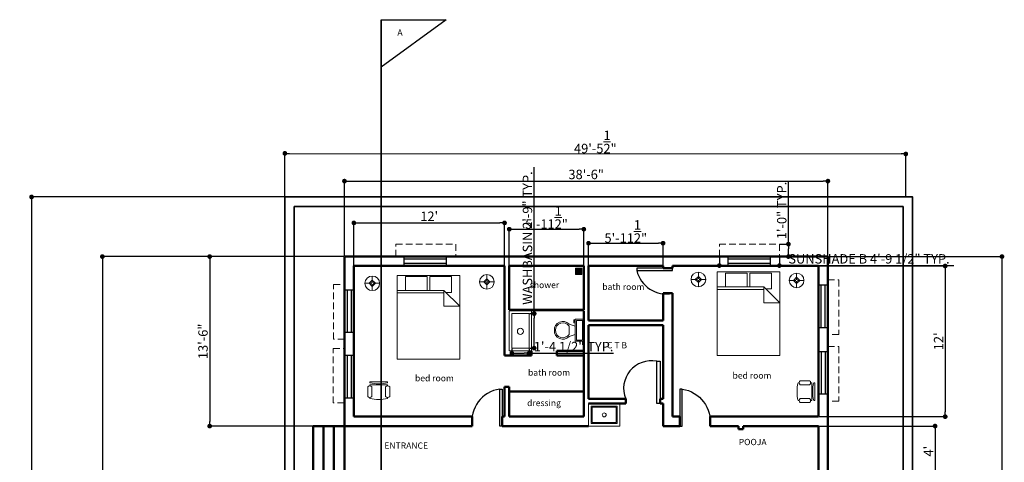
# Model space of a CAD drawing. Units: inches. Extents: x 2050 to 6806, y 2092 to 5743.
# Tile 3 of 8: x 2050 to 2991, y 2706 to 3129. Entities that reach past the tile are written whole.
import ezdxf

# ---------------------------------------------------------------- set-up
doc = ezdxf.new("R2010")
doc.units = ezdxf.units.IN
doc.linetypes.add('HIDDEN', pattern=[9.525, 6.35, -3.175])
for name, color, linetype, lineweight in [('A-ANNO-DIMS', 2, 'Continuous', 18), ('A-ANNO-SYMB', 1, 'Continuous', 25), ('A-AREA-IDEN', 7, 'Continuous', 18), ('A-DOOR', 2, 'Continuous', 25), ('A-FLOR-FIXT', 4, 'Continuous', 18), ('A-FLOR-OVHD', 30, 'HIDDEN', 18), ('A-FURN', 5, 'Continuous', 18), ('A-GLAZ', 6, 'Continuous', 25), ('A-WALL', 7, 'Continuous', 50), ('C-PROP', 90, 'Continuous', 35)]:
    doc.layers.add(name, color=color, linetype=linetype, lineweight=lineweight)
doc.styles.get("Standard").update_dxf_attribs({"font": 'arial.ttf'})
doc.dimstyles.new('ISO-25', dxfattribs={"dimtxt": 9, "dimasz": 4.5, "dimexe": 1.25, "dimexo": 0.625, "dimtad": 1, "dimdec": 1, "dimlunit": 4, "dimtxsty": 'Standard', "dimblk": 'DOT', "dimcen": 2.5, "dimadec": 0, "dimazin": 0, "dimtfac": 1, "dimtdec": 1, "dimtmove": 0, "dimatfit": 3, "dimldrblk": 'ARCHTICK', "dimfxl": 1, "dimarcsym": 0})

# ---------------------------------------------------------------- blocks, each defined once
blk = doc.blocks.new('*U4')
for p, q in [((-10, -8.5), (-8, -8.5)), ((-10, -9.5), (-10, -8.5)), ((-8, -8.5), (-8, -8)), ((-7, -8), (-7, -9.5)), ((-4, -8), (-6, -14)), ((4, -8), (6, -14)), ((9.5, -6), (9.5, -2)), ((-7, -9.5), (-10, -9.5)), ((4, -14), (-4, -14))]:
    blk.add_line(p, q)
blk.add_lwpolyline([(10.5, -8), (10.5, 0), (-10.5, 0), (-10.5, -8)], close=True)
for points in [[(-9.5, -2), (-9.5, -6)], [(8.5, -1), (-8.5, -1)], [(-8.5, -7), (8.5, -7)]]:
    blk.add_lwpolyline(points)
for centre, radius, start, end in [((-8.625, -1.875), 0.8839, 81.8699, 188.1301), ((-8.625, -6.125), 0.8839, 171.869898, 278.1301), ((8.625, -1.875), 0.8839, 351.8699, 98.1301), ((8.625, -6.125), 0.8839, 261.8699, 8.1301), ((-0.4772, -19.9188), 8.0953, 133.01722, 273.38), ((0.0374, -19.8731), 7.127, 124.50543, 269.7), ((-0.0373, -19.8731), 7.127, 270.3, 55.4946), ((0.4773, -19.9188), 8.0953, 266.62, 46.9828)]:
    blk.add_arc(centre, radius, start, end)
blk = doc.blocks.new('Bed - Queen')
for p, q in [((0, -80.00003), (0, 0)), ((0, 0), (59.99999, 0)), ((59.99999, 0), (59.99999, -80.00003)), ((7.99999, -1.2), (28.79998, -1.2)), ((7.99999, -14.4), (7.99999, -1.2)), ((28.79998, -1.2), (28.79998, -14.4)), ((31.19999, -1.2), (51.99999, -1.2)), ((31.19999, -14.4), (31.19999, -1.2)), ((51.99999, -1.2), (51.99999, -16.4)), ((0, -14.4), (44.8, -14.4)), ((44.8, -16.8), (0, -16.8)), ((59.99999, -29.6), (44.8, -14.4)), ((44.8, -14.4), (44.8, -29.6)), ((51.99999, -16.4), (46.79936, -16.4)), ((44.8, -29.6), (59.99999, -29.6)), ((59.99999, -80.00003), (0, -80.00003))]:
    blk.add_line(p, q)
blk = doc.blocks.new('Lamp - Table')
for p, q in [((-1, 0), (-7, 0)), ((0, 3), (-3, 0)), ((-3, 0), (0, -3)), ((0, 7), (0, 1)), ((3, 0), (0, 3)), ((0, -3), (3, 0)), ((1, 0), (7, 0)), ((0, -1), (0, -7))]:
    blk.add_line(p, q)
for radius in [7, 1]:
    blk.add_circle((0, 0), radius)
blk = doc.blocks.new('Chair - Desk')
for p, q in [((-8.5, 0), (-8.5, -1)), ((-8.5, 0), (8.5, 0)), ((8.5, 0), (8.5, -1)), ((-10.5, -5), (-10.5, -14)), ((-8.5, -3), (-8.5, -4)), ((-8.5, -3), (8.5, -3)), ((-6.5, -14), (-6.5, -5)), ((-2, -3), (-2, -1.9355)), ((2, -1.9576), (2, -3)), ((6.5, -5), (6.5, -14)), ((8.5, -3), (8.5, -4)), ((10.5, -14), (10.5, -5)), ((-8.5, -15), (-8.5, -16)), ((8.5, -15), (8.5, -16))]:
    blk.add_line(p, q)
for centre, radius, start, end in [((-8.5, -6.5), 2.5, 36.8699, 143.1301), ((0, 34.625), 36.625, 256.5803, 283.4197), ((8.5, -6.5), 2.5, 36.8699, 143.1301), ((-8.5, -12.5), 2.5, 216.8699, 323.1301), ((0, 19.625), 36.625, 256.5803, 283.4197), ((8.5, -12.5), 2.5, 216.8699, 323.1301)]:
    blk.add_arc(centre, radius, start, end)
blk = doc.blocks.new('_Dot')
at = {"color": 0, "linetype": 'ByBlock', "lineweight": -2}
blk.add_line((-0.5, 0), (-1, 0), dxfattribs=at)
at = {"color": 0, "linetype": 'ByBlock', "const_width": 0.5}
blk.add_lwpolyline([(-0.25, 0, 1), (0.25, 0, 1)], format="xyb", close=True, dxfattribs=at)
blk = doc.blocks.new('*D25')
at = {"layer": 'A-ANNO-DIMS', "color": 0, "lineweight": -2, "transparency": 16777216}
for p, q in [((2302.91, 2959.86), (2302.95, 3002.13)), ((2307.45, 3000.87), (2891.88, 3000.32)), ((2896.35, 2959.3), (2896.39, 3001.56))]:
    blk.add_line(p, q, dxfattribs=at)
at = {"layer": 'Defpoints', "color": 0, "transparency": 16777216}
for p in [(2896.38, 3000.31), (2302.91, 2959.24), (2896.35, 2958.68)]:
    blk.add_point(p, dxfattribs=at)
at = {"layer": 'A-ANNO-DIMS', "color": 0, "lineweight": -2, "transparency": 16777216, "xscale": 4.5, "yscale": 4.5, "zscale": 4.5}
for p, rotation in [((2302.95, 3000.88), 179.9457856727662), ((2896.38, 3000.31), 359.9457856727663)]:
    blk.add_blockref('_Dot', p, dxfattribs=dict(at, rotation=rotation))
at = {"layer": 'A-ANNO-DIMS', "color": 0, "transparency": 16777216, "insert": (2599.68, 3011.83), "char_height": 9, "attachment_point": 5, "rotation": 359.94579}
blk.add_mtext('49\'-5{\\H1x;\\S1/2;}"', dxfattribs=at)
blk = doc.blocks.new('_ArchTick')
at = {"color": 0, "linetype": 'ByBlock', "const_width": 0.15}
blk.add_lwpolyline([(-0.5, -0.5), (0.5, 0.5)], dxfattribs=at)
blk = doc.blocks.new('*D26')
at = {"layer": 'A-ANNO-DIMS', "color": 0, "lineweight": -2, "transparency": 16777216}
for p, q in [((2359.91, 2902.86), (2359.91, 2975.62)), ((2364.41, 2974.37), (2817.41, 2974.37)), ((2821.91, 2902.86), (2821.91, 2975.62))]:
    blk.add_line(p, q, dxfattribs=at)
at = {"layer": 'Defpoints', "color": 0, "transparency": 16777216}
for p in [(2821.91, 2974.37), (2359.91, 2902.24), (2821.91, 2902.24)]:
    blk.add_point(p, dxfattribs=at)
at = {"layer": 'A-ANNO-DIMS', "color": 0, "lineweight": -2, "transparency": 16777216, "xscale": 4.5, "yscale": 4.5, "zscale": 4.5, "rotation": 180}
blk.add_blockref('_Dot', (2359.91, 2974.37), dxfattribs=at)
at = {"layer": 'A-ANNO-DIMS', "color": 0, "lineweight": -2, "transparency": 16777216, "xscale": 4.5, "yscale": 4.5, "zscale": 4.5}
blk.add_blockref('_Dot', (2821.91, 2974.37), dxfattribs=at)
at = {"layer": 'A-ANNO-DIMS', "color": 0, "transparency": 16777216, "insert": (2590.91, 2979.59), "char_height": 9, "attachment_point": 5}
blk.add_mtext('38\'-6"', dxfattribs=at)
blk = doc.blocks.new('*D27')
at = {"layer": 'A-ANNO-DIMS', "color": 0, "lineweight": -2, "transparency": 16777216}
for p, q in [((2302.28, 2959.24), (2059.63, 2959.24)), ((2060.88, 2954.74), (2060.88, 2243.74)), ((2302.28, 2239.24), (2059.63, 2239.24))]:
    blk.add_line(p, q, dxfattribs=at)
at = {"layer": 'Defpoints', "color": 0, "transparency": 16777216}
for p in [(2302.91, 2959.24), (2060.88, 2239.24), (2302.91, 2239.24)]:
    blk.add_point(p, dxfattribs=at)
at = {"layer": 'A-ANNO-DIMS', "color": 0, "lineweight": -2, "transparency": 16777216, "xscale": 4.5, "yscale": 4.5, "zscale": 4.5}
for p, rotation in [((2060.88, 2959.24), 90), ((2060.88, 2239.24), 270)]:
    blk.add_blockref('_Dot', p, dxfattribs=dict(at, rotation=rotation))
at = {"layer": 'A-ANNO-DIMS', "color": 0, "transparency": 16777216, "insert": (2055.66, 2599.24), "char_height": 9, "attachment_point": 5, "rotation": 90}
blk.add_mtext("60'", dxfattribs=at)
blk = doc.blocks.new('*D28')
at = {"layer": 'A-ANNO-DIMS', "color": 0, "lineweight": -2, "transparency": 16777216}
for p, q in [((2359.28, 2902.24), (2127.3, 2902.24)), ((2128.55, 2897.74), (2128.55, 2372.74)), ((2359.28, 2368.24), (2127.3, 2368.24))]:
    blk.add_line(p, q, dxfattribs=at)
at = {"layer": 'Defpoints', "color": 0, "transparency": 16777216}
for p in [(2359.91, 2902.24), (2128.55, 2368.24), (2359.91, 2368.24)]:
    blk.add_point(p, dxfattribs=at)
at = {"layer": 'A-ANNO-DIMS', "color": 0, "lineweight": -2, "transparency": 16777216, "xscale": 4.5, "yscale": 4.5, "zscale": 4.5}
for p, rotation in [((2128.55, 2902.24), 90), ((2128.55, 2368.24), 270)]:
    blk.add_blockref('_Dot', p, dxfattribs=dict(at, rotation=rotation))
at = {"layer": 'A-ANNO-DIMS', "color": 0, "transparency": 16777216, "insert": (2123.33, 2635.24), "char_height": 9, "attachment_point": 5, "rotation": 90}
blk.add_mtext('44\'-6"', dxfattribs=at)
blk = doc.blocks.new('*D29')
at = {"layer": 'A-ANNO-DIMS', "color": 0, "lineweight": -2, "transparency": 16777216}
for p, q in [((2359.28, 2902.24), (2229.85, 2902.24)), ((2231.1, 2897.74), (2231.1, 2744.74)), ((2359.28, 2740.24), (2229.85, 2740.24))]:
    blk.add_line(p, q, dxfattribs=at)
at = {"layer": 'Defpoints', "color": 0, "transparency": 16777216}
for p in [(2359.91, 2902.24), (2231.1, 2740.24), (2359.91, 2740.24)]:
    blk.add_point(p, dxfattribs=at)
at = {"layer": 'A-ANNO-DIMS', "color": 0, "lineweight": -2, "transparency": 16777216, "xscale": 4.5, "yscale": 4.5, "zscale": 4.5}
for p, rotation in [((2231.1, 2902.24), 90), ((2231.1, 2740.24), 270)]:
    blk.add_blockref('_Dot', p, dxfattribs=dict(at, rotation=rotation))
at = {"layer": 'A-ANNO-DIMS', "color": 0, "transparency": 16777216, "insert": (2225.88, 2821.24), "char_height": 9, "attachment_point": 5, "rotation": 90}
blk.add_mtext('13\'-6"', dxfattribs=at)
blk = doc.blocks.new('*D34')
at = {"layer": 'A-ANNO-DIMS', "color": 0, "lineweight": -2, "transparency": 16777216}
for p, q in [((2822.53, 2902.24), (2989.52, 2902.24)), ((2988.27, 2897.74), (2988.27, 2441.74)), ((2822.53, 2437.24), (2989.52, 2437.24))]:
    blk.add_line(p, q, dxfattribs=at)
at = {"layer": 'Defpoints', "color": 0, "transparency": 16777216}
for p in [(2821.91, 2902.24), (2821.91, 2437.24), (2988.27, 2437.24)]:
    blk.add_point(p, dxfattribs=at)
at = {"layer": 'A-ANNO-DIMS', "color": 0, "lineweight": -2, "transparency": 16777216, "xscale": 4.5, "yscale": 4.5, "zscale": 4.5}
for p, rotation in [((2988.27, 2902.24), 90), ((2988.27, 2437.24), 270)]:
    blk.add_blockref('_Dot', p, dxfattribs=dict(at, rotation=rotation))
at = {"layer": 'A-ANNO-DIMS', "color": 0, "transparency": 16777216, "insert": (2983.05, 2669.74), "char_height": 9, "attachment_point": 5, "rotation": 90}
blk.add_mtext('38\'-9"', dxfattribs=at)
blk = doc.blocks.new('*D36')
at = {"layer": 'A-ANNO-DIMS', "color": 0, "lineweight": -2, "transparency": 16777216}
for p, q in [((2809.63, 2740.24), (2925.62, 2740.24)), ((2924.37, 2735.74), (2924.37, 2696.74)), ((2813.53, 2692.24), (2925.62, 2692.24))]:
    blk.add_line(p, q, dxfattribs=at)
at = {"layer": 'Defpoints', "color": 0, "transparency": 16777216}
for p in [(2809.01, 2740.24), (2812.91, 2692.24), (2924.37, 2692.24)]:
    blk.add_point(p, dxfattribs=at)
at = {"layer": 'A-ANNO-DIMS', "color": 0, "lineweight": -2, "transparency": 16777216, "xscale": 4.5, "yscale": 4.5, "zscale": 4.5}
for p, rotation in [((2924.37, 2740.24), 90), ((2924.37, 2692.24), 270)]:
    blk.add_blockref('_Dot', p, dxfattribs=dict(at, rotation=rotation))
at = {"layer": 'A-ANNO-DIMS', "color": 0, "transparency": 16777216, "insert": (2919.24, 2716.24), "char_height": 9, "attachment_point": 5, "rotation": 90}
blk.add_mtext("4'", dxfattribs=at)
blk = doc.blocks.new('*D37')
at = {"layer": 'A-ANNO-DIMS', "color": 0, "lineweight": -2, "transparency": 16777216}
for p, q in [((2813.53, 2893.24), (2935.29, 2893.24)), ((2934.04, 2888.74), (2934.04, 2753.74)), ((2813.53, 2749.24), (2935.29, 2749.24))]:
    blk.add_line(p, q, dxfattribs=at)
at = {"layer": 'Defpoints', "color": 0, "transparency": 16777216}
for p in [(2812.91, 2893.24), (2812.91, 2749.24), (2934.04, 2749.24)]:
    blk.add_point(p, dxfattribs=at)
at = {"layer": 'A-ANNO-DIMS', "color": 0, "lineweight": -2, "transparency": 16777216, "xscale": 4.5, "yscale": 4.5, "zscale": 4.5}
for p, rotation in [((2934.04, 2893.24), 90), ((2934.04, 2749.24), 270)]:
    blk.add_blockref('_Dot', p, dxfattribs=dict(at, rotation=rotation))
at = {"layer": 'A-ANNO-DIMS', "color": 0, "transparency": 16777216, "insert": (2928.9, 2821.24), "char_height": 9, "attachment_point": 5, "rotation": 90}
blk.add_mtext("12'", dxfattribs=at)
blk = doc.blocks.new('*D38')
at = {"layer": 'A-ANNO-DIMS', "color": 0, "lineweight": -2, "transparency": 16777216}
for p, q in [((2593.16, 2893.86), (2593.16, 2916.28)), ((2597.66, 2915.03), (2659.91, 2915.03)), ((2664.41, 2893.86), (2664.41, 2916.28))]:
    blk.add_line(p, q, dxfattribs=at)
at = {"layer": 'Defpoints', "color": 0, "transparency": 16777216}
for p in [(2664.41, 2915.03), (2593.16, 2893.24), (2664.41, 2893.24)]:
    blk.add_point(p, dxfattribs=at)
at = {"layer": 'A-ANNO-DIMS', "color": 0, "lineweight": -2, "transparency": 16777216, "xscale": 4.5, "yscale": 4.5, "zscale": 4.5, "rotation": 180}
blk.add_blockref('_Dot', (2593.16, 2915.03), dxfattribs=at)
at = {"layer": 'A-ANNO-DIMS', "color": 0, "lineweight": -2, "transparency": 16777216, "xscale": 4.5, "yscale": 4.5, "zscale": 4.5}
blk.add_blockref('_Dot', (2664.41, 2915.03), dxfattribs=at)
at = {"layer": 'A-ANNO-DIMS', "color": 0, "transparency": 16777216, "insert": (2628.78, 2926.27), "char_height": 9, "attachment_point": 5}
blk.add_mtext('5\'-11{\\H1x;\\S1/2;}"', dxfattribs=at)
blk = doc.blocks.new('*D39')
at = {"layer": 'A-ANNO-DIMS', "color": 0, "lineweight": -2, "transparency": 16777216}
for p, q in [((2517.41, 2893.86), (2517.41, 2929.65)), ((2521.91, 2928.4), (2584.16, 2928.4)), ((2588.66, 2893.86), (2588.66, 2929.65))]:
    blk.add_line(p, q, dxfattribs=at)
at = {"layer": 'Defpoints', "color": 0, "transparency": 16777216}
for p in [(2588.66, 2928.4), (2517.41, 2893.24), (2588.66, 2893.24)]:
    blk.add_point(p, dxfattribs=at)
at = {"layer": 'A-ANNO-DIMS', "color": 0, "lineweight": -2, "transparency": 16777216, "xscale": 4.5, "yscale": 4.5, "zscale": 4.5, "rotation": 180}
blk.add_blockref('_Dot', (2517.41, 2928.4), dxfattribs=at)
at = {"layer": 'A-ANNO-DIMS', "color": 0, "lineweight": -2, "transparency": 16777216, "xscale": 4.5, "yscale": 4.5, "zscale": 4.5}
blk.add_blockref('_Dot', (2588.66, 2928.4), dxfattribs=at)
at = {"layer": 'A-ANNO-DIMS', "color": 0, "transparency": 16777216, "insert": (2553.03, 2939.64), "char_height": 9, "attachment_point": 5}
blk.add_mtext('5\'-11{\\H1x;\\S1/2;}"', dxfattribs=at)
blk = doc.blocks.new('*D40')
at = {"layer": 'A-ANNO-DIMS', "color": 0, "lineweight": -2, "transparency": 16777216}
for p, q in [((2368.91, 2893.86), (2368.91, 2935.69)), ((2373.41, 2934.44), (2508.41, 2934.44)), ((2512.91, 2893.86), (2512.91, 2935.69))]:
    blk.add_line(p, q, dxfattribs=at)
at = {"layer": 'Defpoints', "color": 0, "transparency": 16777216}
for p in [(2512.91, 2934.44), (2368.91, 2893.24), (2512.91, 2893.24)]:
    blk.add_point(p, dxfattribs=at)
at = {"layer": 'A-ANNO-DIMS', "color": 0, "lineweight": -2, "transparency": 16777216, "xscale": 4.5, "yscale": 4.5, "zscale": 4.5, "rotation": 180}
blk.add_blockref('_Dot', (2368.91, 2934.44), dxfattribs=at)
at = {"layer": 'A-ANNO-DIMS', "color": 0, "lineweight": -2, "transparency": 16777216, "xscale": 4.5, "yscale": 4.5, "zscale": 4.5}
blk.add_blockref('_Dot', (2512.91, 2934.44), dxfattribs=at)
at = {"layer": 'A-ANNO-DIMS', "color": 0, "transparency": 16777216, "insert": (2440.91, 2939.58), "char_height": 9, "attachment_point": 5}
blk.add_mtext("12'", dxfattribs=at)
blk = doc.blocks.new('DOOR-750')
blk.add_lwpolyline([(28.97, 0), (26.83, 0), (26.83, 35.38), (28.97, 35.38)], close=True)
blk.add_arc((31.25, 4.42), 31.27, 98.12333, 188.12333)
blk = doc.blocks.new('DOOR-700')
blk.add_lwpolyline([(34.15, 24.67), (0, 24.67), (0, 22.42), (34.15, 22.42)], close=True)
blk.add_arc((27.99, 28.69), 28.69, 192.63157, 282.38301)
blk = doc.blocks.new('DOOR-900')
blk.add_lwpolyline([(34.8, 0), (31.58, 0), (31.58, 40.43), (34.8, 40.43)], close=True)
blk.add_arc((26.4, 14.55), 26.4, 78.67085, 202.36359)
blk = doc.blocks.new('WIN-1050')
for p, q in [((0, 40.58), (9, 40.58)), ((2.5, 0), (2.5, 40.58)), ((6.5, 0), (6.5, 40.58)), ((0, 0), (9, 0))]:
    blk.add_line(p, q)
blk = doc.blocks.new('SUNSHADE-A')
for p, q in [((0, 52.08), (10.45, 52.08)), ((10.45, 52.08), (10.45, 0)), ((10.45, 0), (0, 0))]:
    blk.add_line(p, q)
blk = doc.blocks.new('SUNSHADE-B')
for p, q in [((0, 0), (0, 11.94)), ((0, 11.94), (57.41, 11.94)), ((57.41, 11.94), (57.41, 0.04))]:
    blk.add_line(p, q)
blk = doc.blocks.new('FLOOR-DRAIN')
blk.add_lwpolyline([(0, 0), (6, 0), (6, 6), (0, 6)], close=True)
for centre in [(0.84, 5.43), (0.84, 4.34), (0.84, 3.14), (0.84, 1.97), (0.84, 0.74), (1.9, 5.43), (2.07, 4.34), (2.07, 3.14), (2.07, 1.97), (2.07, 0.74), (3.09, 5.43), (3.3, 4.34), (3.3, 3.14), (3.3, 1.97), (3.3, 0.74), (4.24, 5.43), (4.49, 4.34), (4.49, 3.14), (4.49, 1.97), (4.49, 0.74), (5.33, 5.43), (5.5, 4.34), (5.5, 3.14), (5.5, 1.97), (5.5, 0.74)]:
    blk.add_circle(centre, 0.471)
blk = doc.blocks.new('WASHBASIN')
blk.add_lwpolyline([(16.37, 33), (16.37, 0), (0, 0), (0, 33)], close=True)
blk.add_circle((8.19, 16.05), 2.91)
blk = doc.blocks.new('*D81')
at = {"layer": 'A-ANNO-DIMS', "color": 0, "lineweight": -2, "transparency": 16777216}
for p, q in [((2718.18, 2901.61), (2718.18, 2892.38)), ((2775.58, 2901.61), (2775.58, 2892.38)), ((2722.68, 2893.63), (2771.08, 2893.63)), ((2775.58, 2893.63), (2942.36, 2893.63))]:
    blk.add_line(p, q, dxfattribs=at)
at = {"layer": 'Defpoints', "color": 0, "transparency": 16777216}
for p in [(2718.18, 2902.24), (2775.58, 2902.24), (2775.58, 2893.63)]:
    blk.add_point(p, dxfattribs=at)
at = {"layer": 'A-ANNO-DIMS', "color": 0, "lineweight": -2, "transparency": 16777216, "xscale": 4.5, "yscale": 4.5, "zscale": 4.5, "rotation": 180}
blk.add_blockref('_Dot', (2718.18, 2893.63), dxfattribs=at)
at = {"layer": 'A-ANNO-DIMS', "color": 0, "lineweight": -2, "transparency": 16777216, "xscale": 4.5, "yscale": 4.5, "zscale": 4.5}
blk.add_blockref('_Dot', (2775.58, 2893.63), dxfattribs=at)
at = {"layer": 'A-ANNO-DIMS', "color": 0, "transparency": 16777216, "insert": (2861.22, 2898.9), "char_height": 9, "attachment_point": 5}
blk.add_mtext('SUNSHADE B 4\'-9 1/2" TYP.', dxfattribs=at)
blk = doc.blocks.new('*D82')
at = {"layer": 'A-ANNO-DIMS', "color": 0, "lineweight": -2, "transparency": 16777216}
for p, q in [((2784.2, 2914.18), (2784.2, 2973.94)), ((2776.21, 2914.18), (2785.45, 2914.18)), ((2784.2, 2906.74), (2784.2, 2909.68)), ((2776.21, 2902.24), (2785.45, 2902.24))]:
    blk.add_line(p, q, dxfattribs=at)
at = {"layer": 'Defpoints', "color": 0, "transparency": 16777216}
for p in [(2775.58, 2914.18), (2784.2, 2914.18), (2775.58, 2902.24)]:
    blk.add_point(p, dxfattribs=at)
at = {"layer": 'A-ANNO-DIMS', "color": 0, "lineweight": -2, "transparency": 16777216, "xscale": 4.5, "yscale": 4.5, "zscale": 4.5}
for p, rotation in [((2784.2, 2914.18), 90), ((2784.2, 2902.24), 270)]:
    blk.add_blockref('_Dot', p, dxfattribs=dict(at, rotation=rotation))
at = {"layer": 'A-ANNO-DIMS', "color": 0, "transparency": 16777216, "insert": (2778.97, 2946.31), "char_height": 9, "attachment_point": 5, "rotation": 90}
blk.add_mtext('1\'-0" TYP.', dxfattribs=at)
blk = doc.blocks.new('*D103')
at = {"layer": 'A-ANNO-DIMS', "color": 0, "lineweight": -2, "transparency": 16777216}
for p, q in [((2541.23, 2847.74), (2541.23, 2987.66)), ((2536.91, 2847.74), (2542.48, 2847.74)), ((2541.23, 2819.24), (2541.23, 2843.24)), ((2536.91, 2814.74), (2542.48, 2814.74))]:
    blk.add_line(p, q, dxfattribs=at)
at = {"layer": 'Defpoints', "color": 0, "transparency": 16777216}
for p in [(2536.28, 2847.74), (2541.23, 2847.74), (2536.28, 2814.74)]:
    blk.add_point(p, dxfattribs=at)
at = {"layer": 'A-ANNO-DIMS', "color": 0, "lineweight": -2, "transparency": 16777216, "xscale": 4.5, "yscale": 4.5, "zscale": 4.5}
for p, rotation in [((2541.23, 2847.74), 90), ((2541.23, 2814.74), 270)]:
    blk.add_blockref('_Dot', p, dxfattribs=dict(at, rotation=rotation))
at = {"layer": 'A-ANNO-DIMS', "color": 0, "transparency": 16777216, "insert": (2535.96, 2919.95), "char_height": 9, "attachment_point": 5, "rotation": 90}
blk.add_mtext('WASHBASIN 2\'-9" TYP.', dxfattribs=at)
blk = doc.blocks.new('*D104')
at = {"layer": 'A-ANNO-DIMS', "color": 0, "lineweight": -2, "transparency": 16777216}
for p, q in [((2519.91, 2814.11), (2519.91, 2808.54)), ((2536.28, 2814.11), (2536.28, 2808.54)), ((2524.41, 2809.79), (2531.78, 2809.79)), ((2536.28, 2809.79), (2617.02, 2809.79))]:
    blk.add_line(p, q, dxfattribs=at)
at = {"layer": 'Defpoints', "color": 0, "transparency": 16777216}
for p in [(2519.91, 2814.74), (2536.28, 2814.74), (2536.28, 2809.79)]:
    blk.add_point(p, dxfattribs=at)
at = {"layer": 'A-ANNO-DIMS', "color": 0, "lineweight": -2, "transparency": 16777216, "xscale": 4.5, "yscale": 4.5, "zscale": 4.5, "rotation": 180}
blk.add_blockref('_Dot', (2519.91, 2809.79), dxfattribs=at)
at = {"layer": 'A-ANNO-DIMS', "color": 0, "lineweight": -2, "transparency": 16777216, "xscale": 4.5, "yscale": 4.5, "zscale": 4.5}
blk.add_blockref('_Dot', (2536.28, 2809.79), dxfattribs=at)
at = {"layer": 'A-ANNO-DIMS', "color": 0, "transparency": 16777216, "insert": (2578.9, 2815.07), "char_height": 9, "attachment_point": 5}
blk.add_mtext('1\'-4 1/2" TYP.', dxfattribs=at)

msp = doc.modelspace()

# ---------------------------------------------------------------- linework, layer by layer
at = {"layer": 'A-ANNO-SYMB'}
for p, q in [((2395, 3128.67), (2395, 2091.98)), ((2395, 2307.82), (2395, 3128.67)), ((2395, 3128.67), (2456.98, 3128.67)), ((2456.98, 3128.67), (2395, 3083.13)), ((2456.98, 3128.67), (2456.98, 3128.67))]:
    msp.add_line(p, q, dxfattribs=at)
at = {"layer": 'A-FLOR-FIXT'}
for p, q in [((2593.16, 2761.69), (2593.16, 2740.24)), ((2620.66, 2759.19), (2595.66, 2759.19)), ((2595.66, 2759.19), (2595.66, 2742.74)), ((2619.66, 2758.19), (2596.66, 2758.19)), ((2596.66, 2758.19), (2596.66, 2743.74)), ((2619.66, 2758.19), (2619.66, 2743.74)), ((2620.66, 2759.19), (2620.66, 2742.74)), ((2623.16, 2761.69), (2623.16, 2740.24)), ((2593.16, 2740.24), (2623.16, 2740.24)), ((2595.66, 2742.74), (2620.66, 2742.74)), ((2596.66, 2743.74), (2619.66, 2743.74))]:
    msp.add_line(p, q, dxfattribs=at)
msp.add_lwpolyline([(2538.78, 2850.24), (2538.78, 2812.24), (2517.41, 2812.24), (2517.41, 2850.24), (2588.66, 2850.24)], dxfattribs=at)
msp.add_circle((2608.16, 2750.97), 1.9, dxfattribs=at)
at = {"layer": 'A-WALL'}
for p, q in [((2821.91, 2902.24), (2359.91, 2902.24)), ((2359.91, 2902.24), (2359.91, 2740.24)), ((2821.91, 2437.24), (2821.91, 2902.24)), ((2368.91, 2893.24), (2368.91, 2749.24)), ((2512.91, 2893.24), (2368.91, 2893.24)), ((2512.91, 2893.24), (2512.91, 2807.74)), ((2517.41, 2893.24), (2517.41, 2851.24)), ((2588.66, 2893.24), (2517.41, 2893.24)), ((2588.66, 2893.24), (2588.66, 2851.24)), ((2664.41, 2893.24), (2593.16, 2893.24)), ((2593.16, 2893.24), (2593.16, 2841.26)), ((2664.41, 2891.25), (2664.41, 2893.24)), ((2664.41, 2891.25), (2673.41, 2891.25)), ((2812.91, 2893.24), (2673.41, 2893.24)), ((2673.41, 2891.25), (2673.41, 2893.24)), ((2812.91, 2749.24), (2812.91, 2893.24)), ((2664.41, 2841.26), (2664.41, 2867.25)), ((2664.41, 2867.25), (2673.41, 2867.25)), ((2673.41, 2749.24), (2673.41, 2867.25)), ((2588.66, 2851.24), (2517.41, 2851.24)), ((2588.66, 2850.24), (2588.66, 2749.24)), ((2664.41, 2841.26), (2593.16, 2841.26)), ((2593.16, 2836.76), (2593.16, 2766.19)), ((2664.41, 2836.76), (2593.16, 2836.76)), ((2593.16, 2836.76), (2593.16, 2826.56)), ((2664.41, 2816.39), (2664.41, 2836.76)), ((2664.41, 2826.56), (2664.41, 2836.76)), ((2664.41, 2826.56), (2664.41, 2836.76)), ((2664.41, 2766.19), (2664.41, 2822.06)), ((2673.41, 2749.24), (2673.41, 2822.06)), ((2538.78, 2807.74), (2512.91, 2807.74)), ((2538.78, 2812.24), (2538.78, 2807.74)), ((2588.66, 2812.24), (2562.78, 2812.24)), ((2562.78, 2812.24), (2562.78, 2807.74)), ((2588.66, 2807.74), (2562.78, 2807.74)), ((2517.41, 2777.74), (2512.91, 2777.74)), ((2512.91, 2777.74), (2512.91, 2749.24)), ((2517.41, 2777.74), (2517.41, 2749.24)), ((2588.66, 2773.24), (2517.41, 2773.24)), ((2628.71, 2766.19), (2593.16, 2766.19)), ((2628.71, 2761.69), (2593.16, 2761.69)), ((2628.71, 2766.19), (2628.71, 2761.69)), ((2664.41, 2766.19), (2661.52, 2766.19)), ((2661.52, 2766.19), (2661.52, 2761.69)), ((2664.41, 2761.69), (2661.52, 2761.69)), ((2664.41, 2740.24), (2664.41, 2761.69)), ((2481.86, 2749.24), (2368.91, 2749.24)), ((2481.86, 2749.24), (2481.86, 2740.24)), ((2481.86, 2749.24), (2481.86, 2740.24)), ((2481.86, 2749.24), (2481.86, 2740.24)), ((2512.91, 2749.24), (2510.54, 2749.24)), ((2510.54, 2749.24), (2510.54, 2740.24)), ((2510.54, 2749.24), (2510.54, 2740.24)), ((2588.66, 2749.24), (2517.41, 2749.24)), ((2680.41, 2749.24), (2673.41, 2749.24)), ((2680.41, 2749.24), (2680.41, 2740.24)), ((2812.91, 2749.24), (2709.4, 2749.24)), ((2709.4, 2749.24), (2709.4, 2740.24)), ((2329.91, 2692.24), (2329.91, 2740.24)), ((2329.91, 2740.24), (2359.91, 2740.24)), ((2339.91, 2692.24), (2339.91, 2740.24)), ((2349.91, 2692.24), (2349.91, 2740.24)), ((2481.86, 2740.24), (2359.91, 2740.24)), ((2359.91, 2692.24), (2359.91, 2740.24)), ((2593.16, 2740.24), (2510.54, 2740.24)), ((2680.41, 2740.24), (2664.41, 2740.24)), ((2736.41, 2740.24), (2709.4, 2740.24)), ((2736.41, 2737.24), (2736.41, 2740.24)), ((2812.91, 2740.24), (2740.91, 2740.24)), ((2740.91, 2737.24), (2740.91, 2740.24)), ((2812.91, 2567.74), (2812.91, 2740.24)), ((2740.91, 2737.24), (2736.41, 2737.24))]:
    msp.add_line(p, q, dxfattribs=at)
at = {"layer": 'C-PROP'}
for p, q in [((2893.91, 2950.24), (2311.91, 2950.24)), ((2311.91, 2950.24), (2311.91, 2248.24)), ((2893.91, 2248.24), (2893.91, 2950.24))]:
    msp.add_line(p, q, dxfattribs=at)
msp.add_lwpolyline([(2902.91, 2239.24), (2902.91, 2959.24), (2302.91, 2959.24), (2302.91, 2239.24), (2681.02, 2239.24)], dxfattribs=at)

# ---------------------------------------------------------------- block references
at = {"layer": 'A-DOOR'}
for name, p in [('DOOR-700', (2639.26, 2866.58)), ('DOOR-900', (2626.72, 2761.69)), ('DOOR-750', (2481.57, 2740.24))]:
    msp.add_blockref(name, p, dxfattribs=at)
at = {"layer": 'A-DOOR', "extrusion": (0, 0, -1), "zscale": -1}
msp.add_blockref('DOOR-750', (-2709.38, 2740.24), dxfattribs=at)
at = {"layer": 'A-FLOR-FIXT'}
for name, p in [('FLOOR-DRAIN', (2580.79, 2885.18)), ('WASHBASIN', (2519.91, 2814.74))]:
    msp.add_blockref(name, p, dxfattribs=at)
at = {"layer": 'A-FLOR-FIXT', "rotation": 270}
msp.add_blockref('*U4', (2588.51, 2831.78), dxfattribs=at)
at = {"layer": 'A-FLOR-OVHD'}
for name, p in [('SUNSHADE-B', (2409.08, 2902.24)), ('SUNSHADE-B', (2718.18, 2902.24)), ('SUNSHADE-A', (2821.91, 2827.86)), ('SUNSHADE-A', (2821.91, 2764.12))]:
    msp.add_blockref(name, p, dxfattribs=at)
at = {"layer": 'A-FLOR-OVHD', "rotation": 180}
for p in [(2359.82, 2875.44), (2359.47, 2814.39)]:
    msp.add_blockref('SUNSHADE-A', p, dxfattribs=at)
at = {"layer": 'A-FURN'}
for name, p in [('Lamp - Table', (2386.53, 2876.68)), ('Bed - Queen', (2410.21, 2884.3)), ('Lamp - Table', (2495.99, 2878.09)), ('Lamp - Table', (2698.12, 2880.35)), ('Bed - Queen', (2716.06, 2887.66)), ('Lamp - Table', (2792.04, 2879.42)), ('Chair - Desk', (2392.64, 2782.62))]:
    msp.add_blockref(name, p, dxfattribs=at)
at = {"layer": 'A-FURN', "rotation": 270}
msp.add_blockref('Chair - Desk', (2809.43, 2773.14), dxfattribs=at)
at = {"layer": 'A-GLAZ'}
for p, rotation in [((2457.41, 2893.28), 90.00000000000124), ((2767.21, 2893.16), 90.00000000000095), ((2368.93, 2870.12), 180), ((2368.93, 2807.57), 180), ((2821.91, 2811.24), 180)]:
    msp.add_blockref('WIN-1050', p, dxfattribs=dict(at, rotation=rotation))
msp.add_blockref('WIN-1050', (2812.91, 2834.5), dxfattribs=at)

# ---------------------------------------------------------------- texts
at = {"layer": 'A-ANNO-SYMB'}
msp.add_text('A', height=6, dxfattribs=at).set_placement((2410.49, 3113.43))
at = {"layer": 'A-AREA-IDEN'}
for s, p in [('shower', (2537.08, 2872.09)), ('bath room', (2606.33, 2870.32)), ('C T B ', (2610.82, 2814.57)), ('bath room', (2535.32, 2788.39)), ('bed room', (2427.3, 2783.03)), ('bed room', (2730.79, 2785.59)), ('dressing ', (2534.44, 2759.32)), ('ENTRANCE', (2398.02, 2718.57)), ('POOJA', (2736.67, 2722))]:
    msp.add_text(s, height=6, dxfattribs=at).set_placement(p)

# ---------------------------------------------------------------- dimensions: what is measured, and where the dimension line sits
at = {"layer": 'A-ANNO-DIMS'}
dim = msp.add_aligned_dim(p1=(2302.91, 2959.24), p2=(2896.35, 2958.68), distance=41.64, dimstyle='ISO-25', override={"dimclrd": 0, "dimclre": 0, "dimclrt": 0}, dxfattribs=at)
dim.commit()
dim.dimension.update_dxf_attribs({"geometry": '*D25', "text_midpoint": (2599.68, 3011.83)})
for base, p1, p2, picture, middle in [((2821.91, 2974.37), (2359.91, 2902.24), (2821.91, 2902.24), '*D26', (2590.91, 2979.59)), ((2512.91, 2934.44), (2368.91, 2893.24), (2512.91, 2893.24), '*D40', (2440.91, 2939.58)), ((2588.6595528, 2928.39647639), (2517.4095528, 2893.23770466), (2588.6595528, 2893.23770466), '*D39', (2553.0345528, 2939.63505075)), ((2664.4095528, 2915.03129049), (2593.1595528, 2893.23770466), (2664.4095528, 2893.23770466), '*D38', (2628.7845528, 2926.26986484))]:
    dim = msp.add_linear_dim(base=base, p1=p1, p2=p2, dimstyle='ISO-25', override={"dimclrd": 0, "dimclre": 0, "dimclrt": 0}, dxfattribs=at)
    dim.commit()
    dim.dimension.update_dxf_attribs({"geometry": picture, "text_midpoint": middle})
for base, p1, p2, text, picture, middle in [((2541.23, 2847.74), (2536.28, 2814.74), (2536.28, 2847.74), 'WASHBASIN <> TYP.', '*D103', (2535.96, 2919.95)), ((2784.2, 2914.18), (2775.58, 2902.24), (2775.58, 2914.18), '<> TYP.', '*D82', (2778.97, 2946.31))]:
    dim = msp.add_linear_dim(base=base, p1=p1, p2=p2, angle=90, text=text, dimstyle='ISO-25', override={"dimdec": 1, "dimlfac": 1, "dimrnd": 0, "dimzin": 1, "dimdsep": 46, "dimlunit": 4, "dimfrac": 2}, dxfattribs=at)
    dim.commit()
    dim.dimension.update_dxf_attribs({"geometry": picture, "text_midpoint": middle})
for base, p1, p2, picture, middle in [((2060.88, 2239.24), (2302.91, 2959.24), (2302.91, 2239.24), '*D27', (2055.66, 2599.24)), ((2128.55, 2368.24), (2359.91, 2902.24), (2359.91, 2368.24), '*D28', (2123.33, 2635.24)), ((2231.1, 2740.24), (2359.91, 2902.24), (2359.91, 2740.24), '*D29', (2225.88, 2821.24)), ((2988.27, 2437.24), (2821.91, 2902.24), (2821.91, 2437.24), '*D34', (2983.05, 2669.74)), ((2934.04, 2749.24), (2812.91, 2893.24), (2812.91, 2749.24), '*D37', (2928.9, 2821.24)), ((2924.37, 2692.24), (2809.01, 2740.24), (2812.91, 2692.24), '*D36', (2919.24, 2716.24))]:
    dim = msp.add_linear_dim(base=base, p1=p1, p2=p2, angle=90, dimstyle='ISO-25', override={"dimclrd": 0, "dimclre": 0, "dimclrt": 0}, dxfattribs=at)
    dim.commit()
    dim.dimension.update_dxf_attribs({"geometry": picture, "text_midpoint": middle})
for base, p1, p2, text, picture, middle in [((2775.58, 2893.63), (2718.18, 2902.24), (2775.58, 2902.24), 'SUNSHADE B <> TYP.', '*D81', (2861.22, 2898.9)), ((2536.28, 2809.79), (2519.91, 2814.74), (2536.28, 2814.74), '<> TYP.', '*D104', (2578.9, 2815.07))]:
    dim = msp.add_linear_dim(base=base, p1=p1, p2=p2, text=text, dimstyle='ISO-25', override={"dimdec": 1, "dimlfac": 1, "dimrnd": 0, "dimzin": 1, "dimdsep": 46, "dimlunit": 4, "dimfrac": 2}, dxfattribs=at)
    dim.commit()
    dim.dimension.update_dxf_attribs({"geometry": picture, "text_midpoint": middle})

doc.saveas('drawing.dxf')
